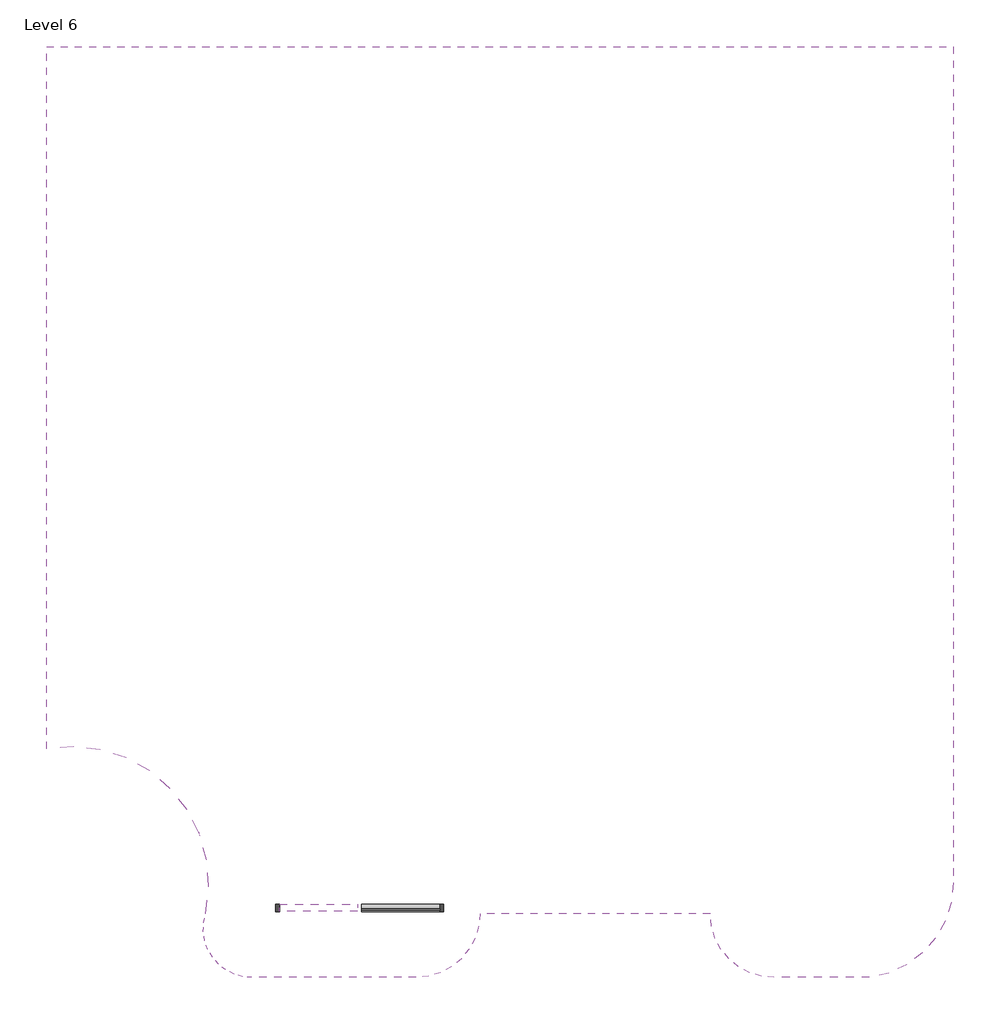
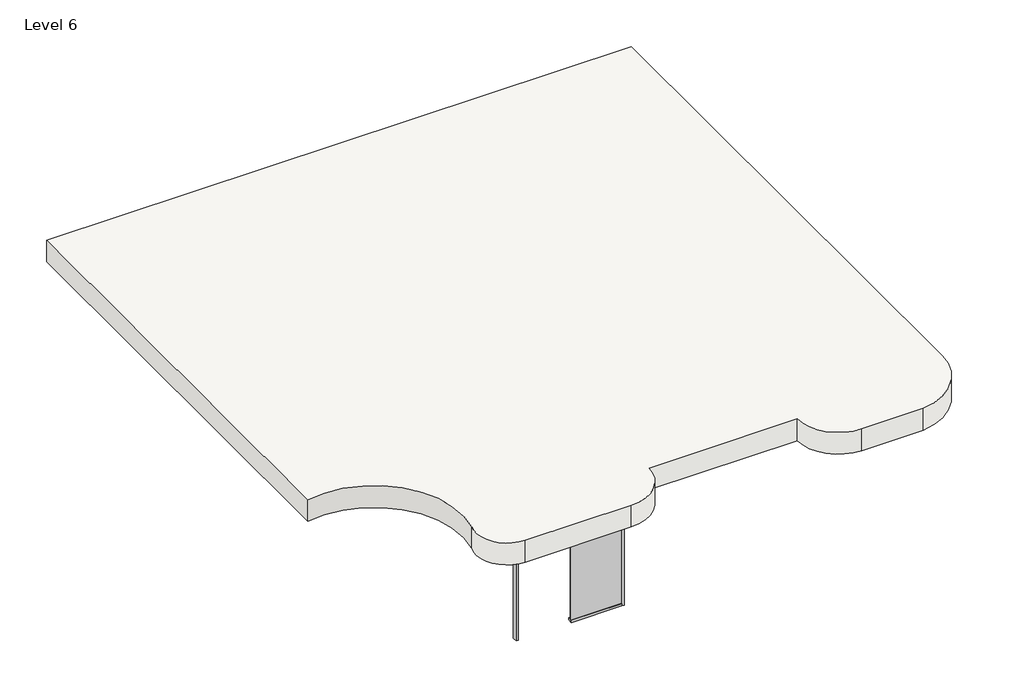
# One storey: 4 members, 1 plate, 1 slab.
"""IFC4 building model written with IfcOpenShell, lengths in millimetres."""

from ifc_helpers import new_model, si_unit, point, frame, frame_2d, origin, place, context, project, spatial, polyline, circle_curve, trimmed, segment, composite_curve, outline, extrude, transform, mapped, element, save
from components import member_3f395ae9, member_0c868e12, system_panel_glazed_7b556abe

model = new_model("IFC4")

# Units and contexts
model_context = context("Model", 3, world=origin())
ifc_project = project(units=[si_unit("LENGTHUNIT", "METRE", prefix="MILLI")], contexts=[model_context])

# Site, building, storey
site = spatial("IfcSite", under=ifc_project)
building = spatial("IfcBuilding", under=site)
storey = spatial("IfcBuildingStorey", under=building, Name="Level 6", Elevation=15240.0)

# Members
placement = place(None, origin())
member_shape = member_3f395ae9(model_context)
element("IfcMember", 1, ObjectType="Rectangular Mullion : 2.5\" x 5\" rectangular", at=placement, inside=storey, context=model_context, shape_type="MappedRepresentation", body=[
    mapped(member_shape, transform((-9111.7115512, -1482.8937024, 14605.0), x_axis=(-1.0, 0.0, 0.0), y_axis=(0.0, 1.0, 0.0), z_axis=(0.0, 0.0, -1.0))),
])
element("IfcMember", 2, ObjectType="Rectangular Mullion : 2.5\" x 5\" rectangular", at=placement, inside=storey, context=model_context, shape_type="MappedRepresentation", body=[
    mapped(member_shape, transform((-6233.4462491, -1482.8937024, 17653.0), x_axis=(1.0, 0.0, 0.0), y_axis=(0.0, 1.0, 0.0), z_axis=(0.0, 0.0, 1.0))),
])
member_2_shape = member_0c868e12(model_context)
element("IfcMember", 3, ObjectType="Rectangular Mullion : 2.5\" x 5\" rectangular", at=placement, inside=storey, context=model_context, shape_type="MappedRepresentation", body=[
    mapped(member_2_shape, transform((-9048.2115512, -1482.8937024, 17653.0), x_axis=(0.0, 0.0, 1.0), y_axis=(0.0, 1.0, 0.0), z_axis=(-1.0, 0.0, 0.0))),
])
element("IfcMember", 4, ObjectType="Rectangular Mullion : 2.5\" x 5\" rectangular", at=placement, inside=storey, context=model_context, shape_type="MappedRepresentation", body=[
    mapped(member_2_shape, transform((-6296.9462491, -1482.8937024, 14605.0), x_axis=(0.0, 0.0, -1.0), y_axis=(0.0, 1.0, 0.0), z_axis=(1.0, 0.0, 0.0))),
])

# Plate
system_panel_glazed_shape = system_panel_glazed_7b556abe(model_context)
element("IfcPlate", 5, ObjectType="System Panel : Glazed", at=placement, inside=storey, context=model_context, shape_type="MappedRepresentation", body=[
    mapped(system_panel_glazed_shape, transform((-6968.8875746, -1482.8937024, 14668.5), x_axis=(-1.0, 0.0, 0.0), y_axis=(0.0, -1.0, 0.0), z_axis=(0.0, 0.0, 1.0))),
])

# Slab
element("IfcSlab", 6, ObjectType="Generic - 2'", at=placement, inside=storey, context=model_context, shape_type="SweptSolid", body=[
    extrude(outline(composite_curve([segment(polyline([(2504.1537509, 13274.5062976), (2504.1537509, -1051.0937024)]), True, "CONTINUOUS"), segment(trimmed(circle_curve(frame_2d((865.9099456, -1051.0937024)), 1638.2438053), [point((2504.1537509, -1051.0937024))], [point((1069.0537509, -2676.6937024))], False, "CARTESIAN"), True, "CONTINUOUS"), segment(polyline([(1069.0537509, -2676.6937024), (-569.2462491, -2676.6937024)]), True, "CONTINUOUS"), segment(trimmed(circle_curve(frame_2d((-569.2462491, -1584.4937024)), 1092.2), [point((-569.2462491, -2676.6937024))], [point((-1661.4462491, -1584.4937024))], False, "CARTESIAN"), True, "CONTINUOUS"), segment(polyline([(-1661.4462491, -1584.4937024), (-5609.8647377, -1584.4937024)]), True, "CONTINUOUS"), segment(trimmed(circle_curve(frame_2d((-6702.0647377, -1584.4937024)), 1092.2), [point((-5609.8647377, -1584.4937024))], [point((-6702.0647377, -2676.6937024))], False, "CARTESIAN"), True, "CONTINUOUS"), segment(polyline([(-6702.0647377, -2676.6937024), (-9521.4647377, -2676.6937024)]), True, "CONTINUOUS"), segment(trimmed(circle_curve(frame_2d((-9521.4647377, -1843.8920375)), 832.801665), [point((-9521.4647377, -2676.6937024))], [point((-10312.8376694, -1584.4937024))], False, "CARTESIAN"), True, "CONTINUOUS"), segment(trimmed(circle_curve(frame_2d((-12612.6150686, -1075.1054509)), 2355.5153315), [point((-10312.8376694, -1584.4937024))], [point((-13040.6462491, 1241.1937063))], True, "CARTESIAN"), True, "CONTINUOUS"), segment(polyline([(-13040.6462491, 1241.1937063), (-13040.6462491, 13274.5062976), (2504.1537509, 13274.5062976)]), True, "CONTINUOUS")], self_intersect=False)), frame((0.0, 0.0, 17653.0), z_axis=(0.0, 0.0, 1.0), x_axis=(1.0, 0.0, 0.0)), (0.0, 0.0, 1.0), 609.6),
])

save(model, "model.ifc")

# Revit data of these elements
# Type "Rectangular Mullion : 2.5\" x 5\" rectangular"
#   built-in parameter 1007304 = 0.416667 (stored number, unit not read)
#   built-in parameter 1007301 = 0.104167 (stored number, unit not read)
#   built-in parameter 1007300 = 0.104167 (stored number, unit not read)
# Type "System Panel : Glazed"
#   Construction Type Id = "GSP4R"
#   Analytic Construction = "1/8 in Pilkington single glazing"
#   Visual Light Transmittance = 0.9
#   Solar Heat Gain Coefficient = 0.86
#   Heat Transfer Coefficient (U) = 1.18115 BTU/(h·ft²·°F)
# Type "Generic - 2'"
#   Assembly Code = "B1010"
#   Function = 0
#   Layers, outside or top first: 2' - 0" no material (function 1)
# Elements 1, 2, 3, 4 (IfcMember, "Rectangular Mullion : 2.5\" x 5\" rectangular")
#   Phase Created = New Construction
#   Materials on its faces: "Iron, Ductile"
# Element 5 (IfcPlate, "System Panel : Glazed")
#   Phase Created = New Construction
#   Materials on its faces: "Glass"
# Element 6 (IfcSlab, "Generic - 2'")
#   Height Offset From Level = 9' - 11"
#   Phase Created = New Construction
#   Materials on its faces: "Default Floor"
# Materials
#   "Iron, Ductile": class "Metal", colour RGB 0 0 0, transparency 0, Description = "Ductile cast iron", Cost = 0
#   "Glass": class "Glass", colour RGB 0 128 192, transparency 0.75, Description = "Soda Lime Glass", Cost = 0
#   "Default Floor": colour RGB 128 128 128, transparency 0
